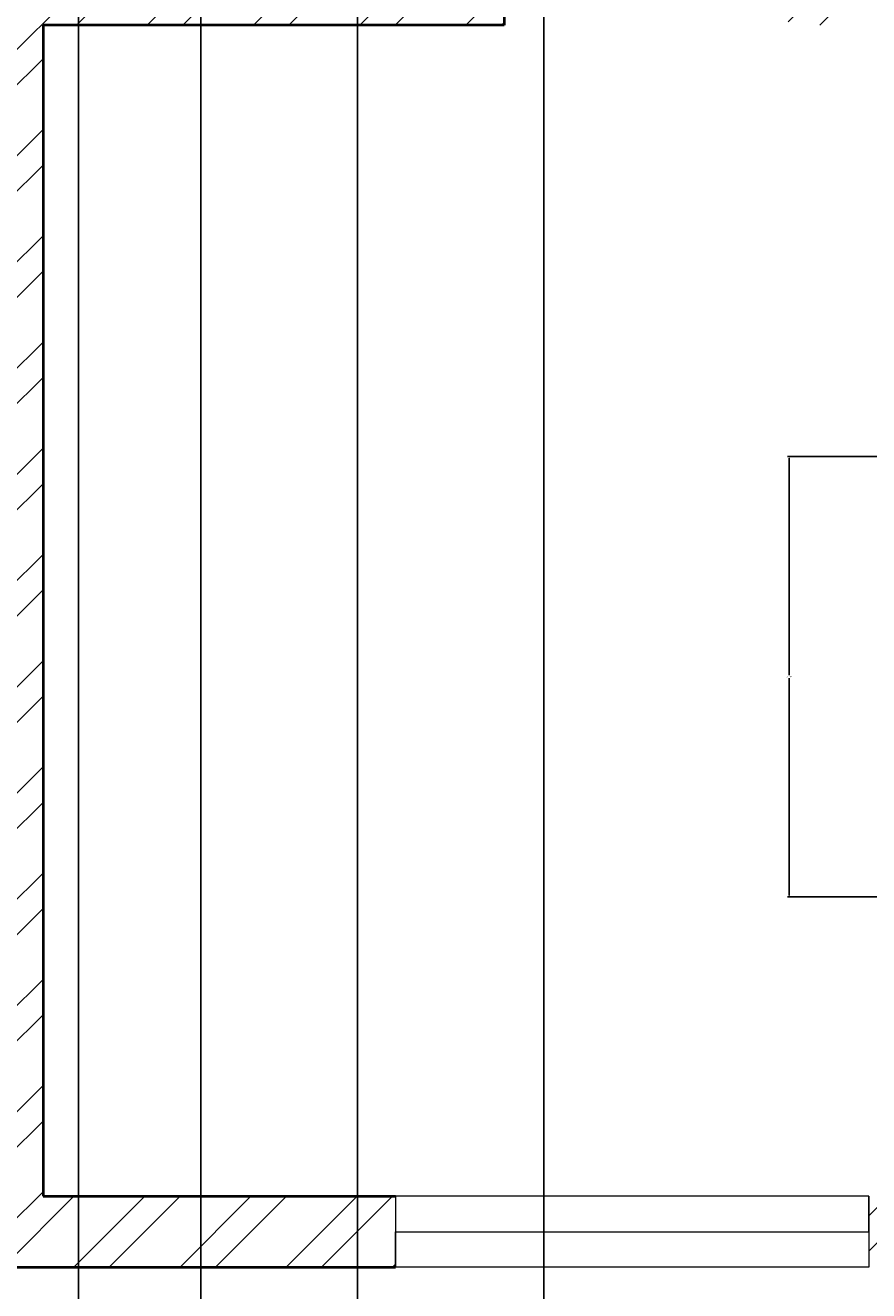
# Model space of a CAD drawing. Units: inches. Extents: x 1601 to 2297, y 1496 to 2631.
# Tile 17 of 57: x 2033 to 2140, y 1632 to 1793. Entities that reach past the tile are written whole.
import ezdxf

# ---------------------------------------------------------------- set-up
doc = ezdxf.new("R2010")
doc.units = ezdxf.units.IN
for name, color, linetype, lineweight in [('A-ANNO-DIMS', 2, 'Continuous', 18), ('A-GLAZ', 161, 'Continuous', 20), ('A-WALL', 7, 'Continuous', 40), ('A-WALL-PATT', 215, 'Continuous', 13)]:
    doc.layers.add(name, color=color, linetype=linetype, lineweight=lineweight)
doc.styles.get("Standard").update_dxf_attribs({"font": 'arial.ttf'})
doc.dimstyles.get("Standard").update_dxf_attribs({"dimtxt": 0.18, "dimasz": 0.18, "dimexe": 0.18, "dimexo": 0.0625, "dimgap": 0.09, "dimtad": 0, "dimtih": 1, "dimtoh": 1, "dimdec": 4, "dimzin": 0, "dimdsep": 46, "dimtxsty": 'Standard', "dimcen": 0.09, "dimadec": 0, "dimazin": 0, "dimtfac": 1, "dimtdec": 4, "dimtofl": 0, "dimtmove": 0, "dimatfit": 3, "dimfxl": 1, "dimtolj": 1, "dimtzin": 0, "dimarcsym": 0})

# ---------------------------------------------------------------- blocks, each defined once
blk = doc.blocks.new('WIN-60IN-JAMB9')
for p, q in [((4.5, 60), (0, 60)), ((0, 60), (9, 60)), ((0, 60), (0, 0)), ((4.5, 0), (4.5, 60)), ((9, 60), (9, 0)), ((0, 0), (9, 0)), ((9, 0), (4.5, 0))]:
    blk.add_line(p, q)
blk = doc.blocks.new('*D13')
at = {"layer": 'A-ANNO-DIMS', "color": 0, "lineweight": -2, "transparency": 16777216}
for p, q in [((2142.32, 1738.13), (2129.97, 1738.13)), ((2130.15, 1737.95), (2130.15, 1710.4)), ((2130.15, 1682.48), (2130.15, 1710.03)), ((2142.32, 1682.3), (2129.97, 1682.3))]:
    blk.add_line(p, q, dxfattribs=at)
at = {"layer": 'A-ANNO-DIMS', "color": 0, "transparency": 16777216}
for points in [[(2130.12, 1737.95), (2130.18, 1737.95), (2130.15, 1738.13)], [(2130.12, 1682.48), (2130.18, 1682.48), (2130.15, 1682.3)]]:
    blk.add_solid(points, dxfattribs=at)
at = {"layer": 'Defpoints', "color": 0, "transparency": 16777216}
for p in [(2142.38, 1738.13), (2130.15, 1682.3), (2142.38, 1682.3)]:
    blk.add_point(p, dxfattribs=at)
at = {"layer": 'A-ANNO-DIMS', "color": 0, "transparency": 16777216, "insert": (2130.15, 1710.22), "char_height": 0.18, "attachment_point": 5}
blk.add_mtext('\\A1;56 TYP.', dxfattribs=at)
blk = doc.blocks.new('*D39')
at = {"layer": 'A-ANNO-DIMS', "color": 0, "lineweight": -2, "transparency": 16777216}
for p, q in [((2055.55, 1981.76), (2055.55, 1513.75)), ((2099.05, 1981.76), (2099.05, 1513.75)), ((2055.73, 1513.93), (2076.97, 1513.93)), ((2098.87, 1513.93), (2077.63, 1513.93))]:
    blk.add_line(p, q, dxfattribs=at)
at = {"layer": 'A-ANNO-DIMS', "color": 0, "transparency": 16777216}
for points in [[(2055.73, 1513.96), (2055.73, 1513.9), (2055.55, 1513.93)], [(2098.87, 1513.96), (2098.87, 1513.9), (2099.05, 1513.93)]]:
    blk.add_solid(points, dxfattribs=at)
at = {"layer": 'Defpoints', "color": 0, "transparency": 16777216}
for p in [(2055.55, 1981.83), (2099.05, 1981.83), (2099.05, 1513.93)]:
    blk.add_point(p, dxfattribs=at)
at = {"layer": 'A-ANNO-DIMS', "color": 0, "transparency": 16777216, "insert": (2077.3, 1513.93), "char_height": 0.18, "attachment_point": 5}
blk.add_mtext('\\A1;43.5', dxfattribs=at)
blk = doc.blocks.new('*D41')
at = {"layer": 'A-ANNO-DIMS', "color": 0, "lineweight": -2, "transparency": 16777216}
for p, q in [((2075.4, 2070.14), (2075.4, 1513.75)), ((2040.04, 2066.51), (2040.04, 1513.75)), ((2040.22, 1513.93), (2057.32, 1513.93)), ((2075.22, 1513.93), (2058.11, 1513.93))]:
    blk.add_line(p, q, dxfattribs=at)
at = {"layer": 'A-ANNO-DIMS', "color": 0, "transparency": 16777216}
for points in [[(2040.22, 1513.96), (2040.22, 1513.9), (2040.04, 1513.93)], [(2075.22, 1513.96), (2075.22, 1513.9), (2075.4, 1513.93)]]:
    blk.add_solid(points, dxfattribs=at)
at = {"layer": 'Defpoints', "color": 0, "transparency": 16777216}
for p in [(2075.4, 2070.2), (2040.04, 2066.58), (2075.4, 1513.93)]:
    blk.add_point(p, dxfattribs=at)
at = {"layer": 'A-ANNO-DIMS', "color": 0, "transparency": 16777216, "insert": (2057.72, 1513.93), "char_height": 0.18, "attachment_point": 5}
blk.add_mtext('\\A1;35.36', dxfattribs=at)

msp = doc.modelspace()

# ---------------------------------------------------------------- hatches: boundary and pattern name
at = {"layer": 'A-WALL-PATT'}
h = msp.add_hatch(dxfattribs=at)
h.set_pattern_fill('ANSI32', color=256)
h.paths.add_polyline_path([(2230.5373, 1861.8254), (2182.5373, 1861.8254), (2182.5373, 1885.3637), (2178.0373, 1885.3637), (2178.0373, 1861.8254), (2166.0373, 1861.8254), (2134.5373, 1861.8254), (2130.0373, 1861.8254), (2130.0373, 1841.4682), (2126.8833, 1841.4682), (2126.8833, 1836.9682), (2130.0373, 1836.9682), (2130.0373, 1822.7302), (2134.5373, 1822.7302), (2134.5373, 1857.3254), (2166.0373, 1857.3254), (2226.0373, 1857.3254), (2226.0373, 1846.1155), (2230.5373, 1846.1155)])
h.paths.add_polyline_path([(2226.0373, 1797.3254), (2134.5373, 1797.3254), (2134.5373, 1800.6636), (2132.2873, 1800.6636), (2130.0373, 1800.6636), (2130.0373, 1797.3254), (2130.0373, 1792.8254), (2167.7264, 1792.8254), (2226.0373, 1792.8254)])
h.paths.add_polyline_path([(2230.5373, 1822.1155), (2226.0373, 1822.1155), (2226.0373, 1760.8563), (2230.5373, 1760.8563)])
h.paths.add_polyline_path([(2230.5373, 1700.8563), (2226.0373, 1700.8563), (2226.0373, 1644.3254), (2140.2517, 1644.3254), (2140.2517, 1635.3254), (2230.5373, 1635.3254)])
h.paths.add_polyline_path([(2080.2517, 1639.8254), (2080.2517, 1644.3254), (2035.5373, 1644.3254), (2035.5373, 1792.8254), (2094.0373, 1792.8254), (2094.0373, 1797.3254), (2094.0373, 1836.9682), (2097.1057, 1836.9682), (2097.1057, 1839.2182), (2097.1057, 1841.4682), (2094.0373, 1841.4682), (2094.0373, 1862.2276), (2089.5373, 1862.2276), (2089.5373, 1797.3254), (2035.5373, 1797.3254), (2035.5373, 1857.3254), (2035.5373, 1885.0916), (2031.0373, 1885.0916), (2031.0373, 1710.3254), (2012.329, 1710.3254), (2012.329, 1701.3254), (2031.0373, 1701.3254), (2031.0373, 1644.3254), (2031.0373, 1635.3254), (2080.2517, 1635.3254)])
h.paths.add_polyline_path([(1836.0373, 1653.2033), (1842.6171, 1653.2033), (1842.6171, 1657.7033), (1842.6171, 1662.2033), (1831.5373, 1662.2033), (1831.5373, 1764.2033), (1835.3881, 1764.2033), (1835.3881, 1766.4533), (1835.3881, 1768.7033), (1831.5373, 1768.7033), (1827.0373, 1768.7033), (1827.0373, 1662.2033), (1827.0373, 1635.3254), (1836.0373, 1635.3254)])
h.paths.add_polyline_path([(1893.0373, 1701.3254), (1907.193, 1701.3254), (1907.193, 1705.8254), (1907.193, 1710.3254), (1893.0373, 1710.3254), (1893.0373, 1819.8254), (1882.6444, 1819.8254), (1882.6444, 1817.5754), (1882.6444, 1815.3254), (1888.5373, 1815.3254), (1888.5373, 1662.2033), (1884.0373, 1662.2033), (1866.6171, 1662.2033), (1866.6171, 1653.2033), (1882.391, 1653.2033), (1884.0373, 1653.2033), (1884.0373, 1635.3254), (1893.0373, 1635.3254)])
h.paths.add_polyline_path([(1739.3335, 1639.8254), (1739.3335, 1644.3254), (1695.0373, 1644.3254), (1695.0373, 1702.0135), (1690.5373, 1702.0135), (1686.0373, 1702.0135), (1686.0373, 1635.3254), (1739.3335, 1635.3254)])
h.paths.add_polyline_path([(1827.0373, 1644.3254), (1799.3335, 1644.3254), (1799.3335, 1635.3254), (1827.0373, 1635.3254)])
h.paths.add_polyline_path([(1695.0373, 1815.3254), (1849.2759, 1815.3254), (1849.2759, 1819.8254), (1807.5373, 1819.8254), (1807.5373, 1879.8254), (1851.1533, 1879.8254), (1851.1533, 1882.0754), (1851.1533, 1884.3254), (1799.3405, 1884.3254), (1799.3405, 1882.0754), (1799.3405, 1879.8254), (1803.0373, 1879.8254), (1803.0373, 1819.8254), (1695.0373, 1819.8254), (1695.0373, 1835.0458), (1690.5373, 1835.0458), (1686.0373, 1835.0458), (1686.0373, 1766.1753), (1695.0373, 1766.1753)])
h.paths.add_polyline_path([(1775.8157, 1884.3254), (1695.0373, 1884.3254), (1695.0373, 1912.9526), (1690.5373, 1912.9526), (1686.0373, 1912.9526), (1686.0373, 1859.0458), (1695.0373, 1859.0458), (1695.0373, 1879.8254), (1775.8157, 1879.8254)])
h.paths.add_polyline_path([(1893.0373, 2031.3254), (1731.5687, 2031.3254), (1731.5687, 2057.4352), (1722.5687, 2057.4352), (1722.5687, 2031.3254), (1686.0373, 2031.3254), (1686.0373, 1972.9526), (1695.0373, 1972.9526), (1695.0373, 2022.3254), (1888.5373, 2022.3254), (1888.5373, 1884.3254), (1883.4996, 1884.3254), (1883.4996, 1879.8254), (1893.0373, 1879.8254), (1893.0373, 1974.3254), (1976.6199, 1974.3254), (1976.6199, 1978.8254), (1968.0373, 1978.8254), (1968.0373, 1983.3254), (1968.0373, 2008.4756), (1963.5373, 2008.4756), (1959.0373, 2008.4756), (1959.0373, 1983.3254), (1893.0373, 1983.3254)])
h.paths.add_polyline_path([(2230.5373, 2140.4745), (2226.0373, 2140.4745), (2226.0373, 2094.3254), (2040.0373, 2094.3254), (2040.0373, 2085.3254), (2178.0373, 2085.3254), (2178.0373, 2065.6965), (2182.5373, 2065.6965), (2182.5373, 2085.3254), (2226.0373, 2085.3254), (2226.0373, 1986.3254), (2211.2679, 1986.3254), (2211.2679, 1981.8254), (2230.5373, 1981.8254)])
h.paths.add_polyline_path([(2187.6292, 1986.3254), (2182.5373, 1986.3254), (2182.5373, 2029.6965), (2178.0373, 2029.6965), (2178.0373, 1986.3254), (2099.05, 1986.3254), (2099.05, 1981.8254), (2178.0373, 1981.8254), (2178.0373, 1969.3637), (2182.5373, 1969.3637), (2182.5373, 1981.8254), (2187.6292, 1981.8254), (2187.6292, 1984.0754)])
h.paths.add_polyline_path([(1807.1169, 1573.5395), (2055.0405, 1573.5395), (2055.0405, 1610.6322), (1807.1169, 1610.6322)], flags=9)
h.paths.add_polyline_path([(1841.1631, 1712.7967), (1870.3957, 1712.7967), (1870.3957, 1731.454), (1841.1631, 1731.454)], flags=9)
h.paths.add_polyline_path([(2144.3862, 1772.185), (2191.0233, 1772.185), (2191.0233, 1790.8423), (2144.3862, 1790.8423)], flags=9)
h.paths.add_polyline_path([(2143.0128, 1827.3312), (2177.9958, 1827.3312), (2177.9958, 1845.9886), (2143.0128, 1845.9886)], flags=25)
h.paths.add_polyline_path([(2041.2439, 1833.5691), (2070.8516, 1833.5691), (2070.8516, 1852.2264), (2041.2439, 1852.2264)], flags=25)
h.paths.add_polyline_path([(2097.2791, 1947.0598), (2134.2061, 1947.0598), (2134.2061, 1965.7171), (2097.2791, 1965.7171)], flags=9)
h.paths.add_polyline_path([(2214.995, 1904.3124), (2214.995, 1942.2899), (2196.3376, 1942.2899), (2196.3376, 1904.3124)], flags=9)
h.paths.add_polyline_path([(2186.6284, 2043.8031), (2219.7935, 2043.8031), (2219.7935, 2062.4605), (2186.6284, 2062.4605)], flags=25)
h.paths.add_polyline_path([(2064.0877, 2031.616), (2097.4949, 2031.616), (2097.4949, 2050.2734), (2064.0877, 2050.2734)], flags=25)
h.paths.add_polyline_path([(1973.1349, 1986.0688), (2008.4009, 1986.0688), (2008.4009, 2004.7261), (1973.1349, 2004.7261)], flags=9)
h.paths.add_polyline_path([(1976.3676, 2106.9635), (2005.7469, 2106.9635), (2005.7469, 2125.6209), (1976.3676, 2125.6209)], flags=9)
h.paths.add_polyline_path([(1991.7852, 2180.4863), (2027.0513, 2180.4863), (2027.0513, 2199.1437), (1991.7852, 2199.1437)], flags=9)
h.paths.add_polyline_path([(2106.1801, 2187.9359), (2152.2101, 2187.9359), (2152.2101, 2206.5932), (2106.1801, 2206.5932)], flags=9)
h.paths.add_polyline_path([(2148.6686, 2262.2542), (2182.318, 2262.2542), (2182.318, 2280.9115), (2148.6686, 2280.9115)], flags=9)
h.paths.add_polyline_path([(2041.6327, 2252.8147), (2071.2405, 2252.8147), (2071.2405, 2271.4721), (2041.6327, 2271.4721)], flags=9)
h.paths.add_polyline_path([(2063.9734, 2375.4265), (2100.9004, 2375.4265), (2100.9004, 2394.0839), (2063.9734, 2394.0839)], flags=9)
h.paths.add_polyline_path([(2216.4955, 2330.9748), (2216.4955, 2370.2654), (2197.8381, 2370.2654), (2197.8381, 2330.9748)], flags=9)
h.paths.add_polyline_path([(2179.1416, 2485.8687), (2212.3067, 2485.8687), (2212.3067, 2504.5261), (2179.1416, 2504.5261)], flags=9)
h.paths.add_polyline_path([(2078.7442, 2471.1516), (2112.1514, 2471.1516), (2112.1514, 2489.809), (2078.7442, 2489.809)], flags=9)
h.paths.add_polyline_path([(1915.9631, 2329.4668), (1952.8902, 2329.4668), (1952.8902, 2348.1241), (1915.9631, 2348.1241)], flags=9)
h.paths.add_polyline_path([(1904.3189, 2499.6709), (1940.4512, 2499.6709), (1940.4512, 2518.3282), (1904.3189, 2518.3282)], flags=9)
h.paths.add_polyline_path([(1892.3665, 2100.4595), (1925.6374, 2100.4595), (1925.6374, 2119.1169), (1892.3665, 2119.1169)], flags=9)
h.paths.add_polyline_path([(1909.2984, 1805.9631), (1946.2254, 1805.9631), (1946.2254, 1824.6205), (1909.2984, 1824.6205)], flags=9)
h.paths.add_polyline_path([(1934.6056, 1658.616), (1970.738, 1658.616), (1970.738, 1677.2733), (1934.6056, 1677.2733)], flags=9)
h.paths.add_polyline_path([(1711.2052, 1789.8902), (1750.0456, 1789.8902), (1750.0456, 1808.5476), (1711.2052, 1808.5476)], flags=25)
h.paths.add_polyline_path([(1742.7874, 1854.6743), (1771.9449, 1854.6743), (1771.9449, 1873.3317), (1742.7874, 1873.3317)], flags=25)
h.paths.add_polyline_path([(1807.3592, 1997.7912), (1850.1116, 1997.7912), (1850.1116, 2016.4486), (1807.3592, 2016.4486)], flags=25)
h.paths.add_polyline_path([(1717.4579, 2237.7844), (1760.2103, 2237.7844), (1760.2103, 2256.4417), (1717.4579, 2256.4417)], flags=9)
h.paths.add_polyline_path([(1780.9285, 2324.0623), (1810.086, 2324.0623), (1810.086, 2342.7197), (1780.9285, 2342.7197)], flags=9)
h.paths.add_polyline_path([(1837.696, 2449.2024), (1866.9286, 2449.2024), (1866.9286, 2467.8598), (1837.696, 2467.8598)], flags=9)
h.paths.add_polyline_path([(1712.7752, 2484.9404), (1751.6156, 2484.9404), (1751.6156, 2503.5977), (1712.7752, 2503.5977)], flags=9)

# ---------------------------------------------------------------- linework, layer by layer
at = {"layer": 'A-WALL'}
for p, q in [((2094.0373, 1797.3254), (2094.0373, 1792.8254)), ((2094.0373, 1792.8254), (2035.5373, 1792.8254)), ((2035.5373, 1792.8254), (2035.5373, 1644.3254)), ((2035.5373, 1644.3254), (2080.2517, 1644.3254)), ((1884.0373, 1635.3254), (2080.2517, 1635.3254))]:
    msp.add_line(p, q, dxfattribs=at)

# ---------------------------------------------------------------- block references
at = {"layer": 'A-GLAZ', "rotation": 269.999999999997}
msp.add_blockref('WIN-60IN-JAMB9', (2080.2512, 1644.3257), dxfattribs=at)

# ---------------------------------------------------------------- dimensions: what is measured, and where the dimension line sits
at = {"layer": 'A-ANNO-DIMS'}
for base, p1, p2, override, picture, middle in [((2075.3977, 1513.9279), (2040.0373, 2066.5754), (2075.3977, 2070.1988), {"dimdec": 2, "dimlfac": 1, "dimrnd": 0, "dimzin": 0, "dimdsep": 46, "dimlunit": 2}, '*D41', (2057.7175, 1513.9279)), ((2099.05, 1513.9279), (2055.5513, 1981.8254), (2099.05, 1981.8254), {"dimdec": 1, "dimlfac": 1, "dimrnd": 0, "dimzin": 0, "dimdsep": 46, "dimlunit": 2}, '*D39', (2077.3006, 1513.9279))]:
    dim = msp.add_linear_dim(base=base, p1=p1, p2=p2, dimstyle='Standard', override=override, dxfattribs=at)
    dim.commit()
    dim.dimension.update_dxf_attribs({"geometry": picture, "text_midpoint": middle})
dim = msp.add_linear_dim(base=(2130.1464, 1682.3035), p1=(2142.3787, 1738.1281), p2=(2142.3787, 1682.3035), angle=270, text='<> TYP.', dimstyle='Standard', override={"dimdec": 0, "dimlfac": 1, "dimrnd": 0, "dimzin": 0, "dimdsep": 46, "dimlunit": 2}, dxfattribs=at)
dim.commit()
dim.dimension.update_dxf_attribs({"geometry": '*D13', "text_midpoint": (2130.1464, 1710.2158)})

doc.saveas('drawing.dxf')
